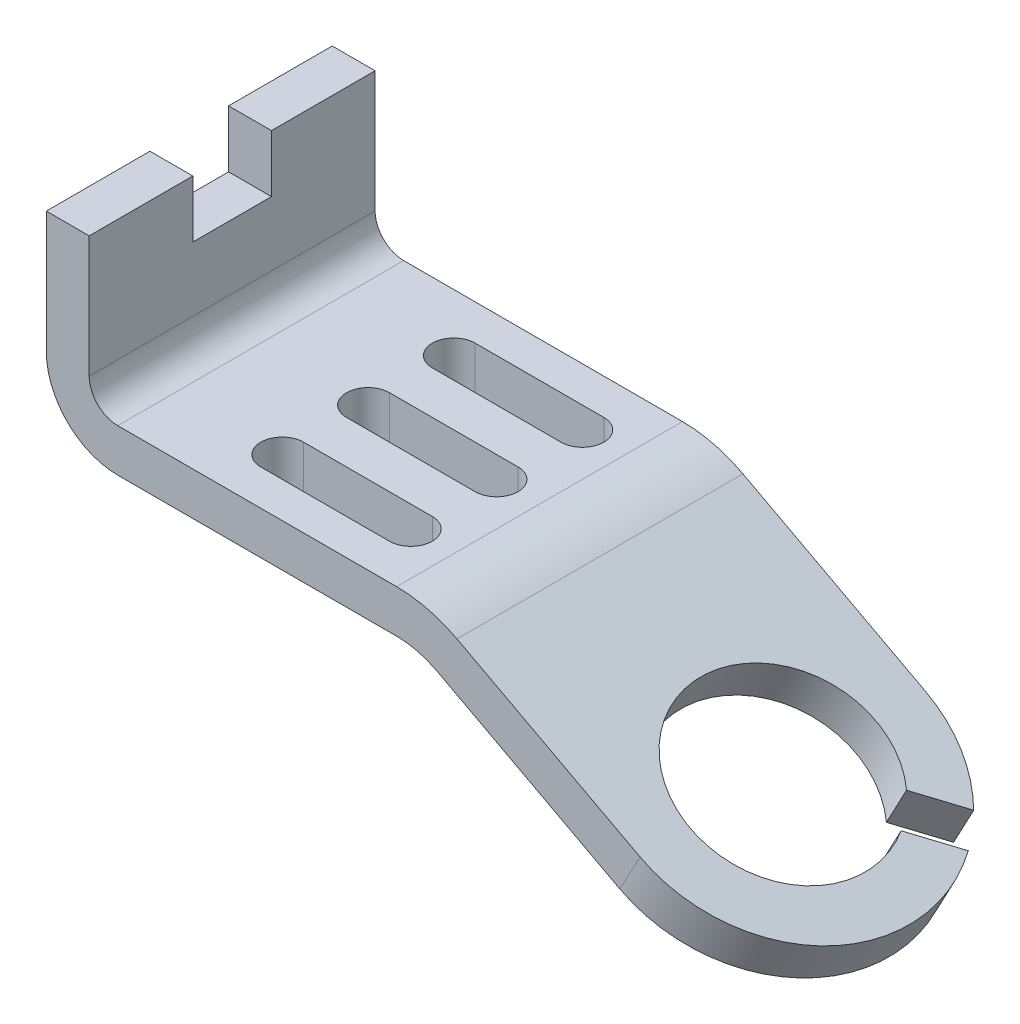
ISO-10303-21;
HEADER;
FILE_DESCRIPTION(('STEP AP214'),'2;1');
FILE_NAME('part.step','',(''),(''),'','','');
FILE_SCHEMA(('AUTOMOTIVE_DESIGN { 1 0 10303 214 1 1 1 1 }'));
ENDSEC;
DATA;
#1=APPLICATION_CONTEXT('core data for automotive mechanical design processes');
#2=APPLICATION_PROTOCOL_DEFINITION('international standard','automotive_design',2000,#1);
#3=PRODUCT_CONTEXT('',#1,'mechanical');
#4=PRODUCT('Part','Part','',(#3));
#5=PRODUCT_RELATED_PRODUCT_CATEGORY('part','',(#4));
#6=PRODUCT_DEFINITION_FORMATION('','',#4);
#7=PRODUCT_DEFINITION_CONTEXT('part definition',#1,'design');
#8=PRODUCT_DEFINITION('design','',#6,#7);
#9=PRODUCT_DEFINITION_SHAPE('','',#8);
#10=(LENGTH_UNIT() NAMED_UNIT(*) SI_UNIT(.MILLI.,.METRE.));
#11=(NAMED_UNIT(*) PLANE_ANGLE_UNIT() SI_UNIT($,.RADIAN.));
#12=(NAMED_UNIT(*) SI_UNIT($,.STERADIAN.) SOLID_ANGLE_UNIT());
#13=UNCERTAINTY_MEASURE_WITH_UNIT(LENGTH_MEASURE(1.E-05),#10,'distance_accuracy_value','');
#14=(GEOMETRIC_REPRESENTATION_CONTEXT(3) GLOBAL_UNCERTAINTY_ASSIGNED_CONTEXT((#13)) GLOBAL_UNIT_ASSIGNED_CONTEXT((#10,
#11,#12)) REPRESENTATION_CONTEXT('',''));
#15=CARTESIAN_POINT('',(0.,0.,0.));
#16=DIRECTION('',(0.,0.,1.));
#17=DIRECTION('',(1.,0.,0.));
#18=AXIS2_PLACEMENT_3D('',#15,#16,#17);
#19=CARTESIAN_POINT('',(0.,27.,40.));
#20=DIRECTION('',(0.,-1.,0.));
#21=DIRECTION('',(0.,0.,-1.));
#22=AXIS2_PLACEMENT_3D('',#19,#20,#21);
#23=PLANE('',#22);
#24=DIRECTION('',(0.,0.,-1.));
#25=VECTOR('',#24,1.);
#26=CARTESIAN_POINT('',(0.,27.,40.));
#27=LINE('',#26,#25);
#28=CARTESIAN_POINT('',(0.,27.,14.5));
#29=VERTEX_POINT('',#28);
#30=CARTESIAN_POINT('',(0.,27.,0.));
#31=VERTEX_POINT('',#30);
#32=EDGE_CURVE('E50',#29,#31,#27,.T.);
#33=ORIENTED_EDGE('',*,*,#32,.F.);
#34=DIRECTION('',(-1.,0.,0.));
#35=VECTOR('',#34,1.);
#36=CARTESIAN_POINT('',(-0.00100000000000013,27.,14.5));
#37=LINE('',#36,#35);
#38=CARTESIAN_POINT('',(6.,27.,14.5));
#39=VERTEX_POINT('',#38);
#40=EDGE_CURVE('E252',#39,#29,#37,.T.);
#41=ORIENTED_EDGE('',*,*,#40,.F.);
#42=DIRECTION('',(0.,0.,-1.));
#43=VECTOR('',#42,1.);
#44=CARTESIAN_POINT('',(6.,27.,40.));
#45=LINE('',#44,#43);
#46=CARTESIAN_POINT('',(6.,27.,0.));
#47=VERTEX_POINT('',#46);
#48=EDGE_CURVE('E264',#39,#47,#45,.T.);
#49=ORIENTED_EDGE('',*,*,#48,.T.);
#50=DIRECTION('',(-1.,0.,0.));
#51=VECTOR('',#50,1.);
#52=CARTESIAN_POINT('',(0.,27.,0.));
#53=LINE('',#52,#51);
#54=EDGE_CURVE('E312',#47,#31,#53,.T.);
#55=ORIENTED_EDGE('',*,*,#54,.T.);
#56=EDGE_LOOP('',(#33,#41,#49,#55));
#57=FACE_BOUND('',#56,.T.);
#58=ADVANCED_FACE('F39',(#57),#23,.F.);
#59=CARTESIAN_POINT('',(54.6417227193125,-1.40462888569289,40.));
#60=DIRECTION('',(0.469471562785892,0.882947592858927,0.));
#61=DIRECTION('',(-0.882947592858927,0.469471562785892,0.));
#62=AXIS2_PLACEMENT_3D('',#59,#60,#61);
#63=PLANE('',#62);
#64=CARTESIAN_POINT('',(80.2472029122214,-15.0193042064837,20.));
#65=DIRECTION('',(0.469471562785892,0.882947592858927,0.));
#66=DIRECTION('',(-0.882947592858927,0.469471562785892,0.));
#67=AXIS2_PLACEMENT_3D('',#64,#65,#66);
#68=CIRCLE('',#67,20.);
#69=CARTESIAN_POINT('',(94.7444514296889,-22.7276279763616,8.580213220838));
#70=VERTEX_POINT('',#69);
#71=CARTESIAN_POINT('',(80.2472029122214,-15.0193042064837,40.));
#72=VERTEX_POINT('',#71);
#73=EDGE_CURVE('E399',#70,#72,#68,.F.);
#74=ORIENTED_EDGE('',*,*,#73,.T.);
#75=DIRECTION('',(0.882947592858927,-0.469471562785892,0.));
#76=VECTOR('',#75,1.);
#77=CARTESIAN_POINT('',(54.6417227193125,-1.40462888569289,40.));
#78=LINE('',#77,#76);
#79=CARTESIAN_POINT('',(54.6417227193125,-1.40462888569288,40.));
#80=VERTEX_POINT('',#79);
#81=EDGE_CURVE('E358',#80,#72,#78,.T.);
#82=ORIENTED_EDGE('',*,*,#81,.F.);
#83=DIRECTION('',(0.,0.,-1.));
#84=VECTOR('',#83,1.);
#85=CARTESIAN_POINT('',(54.6417227193125,-1.40462888569288,40.));
#86=LINE('',#85,#84);
#87=CARTESIAN_POINT('',(54.6417227193125,-1.40462888569288,0.));
#88=VERTEX_POINT('',#87);
#89=EDGE_CURVE('E294',#80,#88,#86,.T.);
#90=ORIENTED_EDGE('',*,*,#89,.T.);
#91=DIRECTION('',(0.882947592858927,-0.469471562785892,0.));
#92=VECTOR('',#91,1.);
#93=CARTESIAN_POINT('',(54.6417227193125,-1.40462888569289,0.));
#94=LINE('',#93,#92);
#95=CARTESIAN_POINT('',(80.2472029122214,-15.0193042064837,0.));
#96=VERTEX_POINT('',#95);
#97=EDGE_CURVE('E332',#88,#96,#94,.T.);
#98=ORIENTED_EDGE('',*,*,#97,.T.);
#99=CARTESIAN_POINT('',(80.2472029122214,-15.0193042064837,20.));
#100=DIRECTION('',(0.469471562785892,0.882947592858927,0.));
#101=DIRECTION('',(-0.882947592858927,0.469471562785892,0.));
#102=AXIS2_PLACEMENT_3D('',#99,#100,#101);
#103=CIRCLE('',#102,20.);
#104=CARTESIAN_POINT('',(91.7904151387249,-21.1569390189858,4.86448909345104));
#105=VERTEX_POINT('',#104);
#106=EDGE_CURVE('E64',#96,#105,#103,.F.);
#107=ORIENTED_EDGE('',*,*,#106,.T.);
#108=DIRECTION('',(-0.656157934800832,0.34888536259312,0.669130606358859));
#109=VECTOR('',#108,1.);
#110=CARTESIAN_POINT('',(49.5631238493171,1.29571003310903,47.9266415521427));
#111=LINE('',#110,#109);
#112=CARTESIAN_POINT('',(87.1410217357462,-18.6848126951173,9.60580404513316));
#113=VERTEX_POINT('',#112);
#114=EDGE_CURVE('E835',#105,#113,#111,.T.);
#115=ORIENTED_EDGE('',*,*,#114,.T.);
#116=CARTESIAN_POINT('',(80.2472029122214,-15.0193042064837,20.));
#117=DIRECTION('',(0.469471562785892,0.882947592858927,0.));
#118=DIRECTION('',(-0.882947592858927,0.469471562785892,0.));
#119=AXIS2_PLACEMENT_3D('',#116,#117,#118);
#120=CIRCLE('',#119,13.);
#121=CARTESIAN_POINT('',(90.0950580267101,-20.2555016524931,13.3215281725201));
#122=VERTEX_POINT('',#121);
#123=EDGE_CURVE('E407',#122,#113,#120,.F.);
#124=ORIENTED_EDGE('',*,*,#123,.F.);
#125=DIRECTION('',(-0.65615793480083,0.34888536259312,0.669130606358861));
#126=VECTOR('',#125,1.);
#127=CARTESIAN_POINT('',(52.5171601402812,-0.274978924266915,51.6423656795297));
#128=LINE('',#127,#126);
#129=EDGE_CURVE('E402',#70,#122,#128,.T.);
#130=ORIENTED_EDGE('',*,*,#129,.F.);
#131=EDGE_LOOP('',(#74,#82,#90,#98,#107,#115,#124,#130));
#132=FACE_BOUND('',#131,.T.);
#133=ADVANCED_FACE('F395',(#132),#63,.F.);
#134=CARTESIAN_POINT('',(57.4585520960279,3.89305667146068,40.));
#135=DIRECTION('',(-0.469471562785892,-0.882947592858927,0.));
#136=DIRECTION('',(0.882947592858926,-0.469471562785892,0.));
#137=AXIS2_PLACEMENT_3D('',#134,#135,#136);
#138=PLANE('',#137);
#139=CARTESIAN_POINT('',(83.0640322889367,-9.72161864933019,20.));
#140=DIRECTION('',(0.469471562785892,0.882947592858926,0.));
#141=DIRECTION('',(-0.882947592858927,0.469471562785892,0.));
#142=AXIS2_PLACEMENT_3D('',#139,#140,#141);
#143=CIRCLE('',#142,20.);
#144=CARTESIAN_POINT('',(83.0640322889367,-9.72161864933019,40.));
#145=VERTEX_POINT('',#144);
#146=CARTESIAN_POINT('',(97.5612808064042,-17.4299424192081,8.58021322083801));
#147=VERTEX_POINT('',#146);
#148=EDGE_CURVE('E401',#145,#147,#143,.T.);
#149=ORIENTED_EDGE('',*,*,#148,.T.);
#150=DIRECTION('',(0.65615793480083,-0.34888536259312,-0.669130606358861));
#151=VECTOR('',#150,1.);
#152=CARTESIAN_POINT('',(55.3339895169966,5.02270663288664,51.6423656795296));
#153=LINE('',#152,#151);
#154=CARTESIAN_POINT('',(92.9118874034255,-14.9578160953396,13.3215281725201));
#155=VERTEX_POINT('',#154);
#156=EDGE_CURVE('E416',#155,#147,#153,.T.);
#157=ORIENTED_EDGE('',*,*,#156,.F.);
#158=CARTESIAN_POINT('',(83.0640322889367,-9.72161864933019,20.));
#159=DIRECTION('',(0.469471562785892,0.882947592858926,0.));
#160=DIRECTION('',(-0.882947592858927,0.469471562785892,0.));
#161=AXIS2_PLACEMENT_3D('',#158,#159,#160);
#162=CIRCLE('',#161,13.);
#163=CARTESIAN_POINT('',(89.9578511124615,-13.3871271379638,9.60580404513316));
#164=VERTEX_POINT('',#163);
#165=EDGE_CURVE('E415',#164,#155,#162,.T.);
#166=ORIENTED_EDGE('',*,*,#165,.F.);
#167=DIRECTION('',(0.656157934800832,-0.348885362593121,-0.669130606358859));
#168=VECTOR('',#167,1.);
#169=CARTESIAN_POINT('',(52.3799532260324,6.59339559026258,47.9266415521427));
#170=LINE('',#169,#168);
#171=CARTESIAN_POINT('',(94.6072445154403,-15.8592534618322,4.86448909345104));
#172=VERTEX_POINT('',#171);
#173=EDGE_CURVE('E412',#164,#172,#170,.T.);
#174=ORIENTED_EDGE('',*,*,#173,.T.);
#175=CARTESIAN_POINT('',(83.0640322889367,-9.72161864933019,0.));
#176=VERTEX_POINT('',#175);
#177=EDGE_CURVE('E408',#172,#176,#143,.T.);
#178=ORIENTED_EDGE('',*,*,#177,.T.);
#179=DIRECTION('',(-0.882947592858927,0.469471562785892,0.));
#180=VECTOR('',#179,1.);
#181=CARTESIAN_POINT('',(57.4585520960279,3.89305667146068,0.));
#182=LINE('',#181,#180);
#183=CARTESIAN_POINT('',(57.4585520960279,3.89305667146068,0.));
#184=VERTEX_POINT('',#183);
#185=EDGE_CURVE('E331',#176,#184,#182,.T.);
#186=ORIENTED_EDGE('',*,*,#185,.T.);
#187=DIRECTION('',(0.,0.,-1.));
#188=VECTOR('',#187,1.);
#189=CARTESIAN_POINT('',(57.4585520960279,3.89305667146068,40.));
#190=LINE('',#189,#188);
#191=CARTESIAN_POINT('',(57.4585520960279,3.89305667146068,40.));
#192=VERTEX_POINT('',#191);
#193=EDGE_CURVE('E292',#192,#184,#190,.T.);
#194=ORIENTED_EDGE('',*,*,#193,.F.);
#195=DIRECTION('',(-0.882947592858927,0.469471562785892,0.));
#196=VECTOR('',#195,1.);
#197=CARTESIAN_POINT('',(57.4585520960279,3.89305667146068,40.));
#198=LINE('',#197,#196);
#199=EDGE_CURVE('E362',#145,#192,#198,.T.);
#200=ORIENTED_EDGE('',*,*,#199,.F.);
#201=EDGE_LOOP('',(#149,#157,#166,#174,#178,#186,#194,#200));
#202=FACE_BOUND('',#201,.T.);
#203=ADVANCED_FACE('F553',(#202),#138,.F.);
#204=CARTESIAN_POINT('',(10.,10.,40.));
#205=DIRECTION('',(0.,0.,1.));
#206=DIRECTION('',(1.,0.,0.));
#207=AXIS2_PLACEMENT_3D('',#204,#205,#206);
#208=PLANE('',#207);
#209=ORIENTED_EDGE('',*,*,#81,.T.);
#210=DIRECTION('',(0.469471562785892,0.882947592858926,0.));
#211=VECTOR('',#210,1.);
#212=CARTESIAN_POINT('',(57.7654060668948,-57.3014145220289,40.));
#213=LINE('',#212,#211);
#214=EDGE_CURVE('E388',#72,#145,#213,.T.);
#215=ORIENTED_EDGE('',*,*,#214,.T.);
#216=ORIENTED_EDGE('',*,*,#199,.T.);
#217=CARTESIAN_POINT('',(49.0080639658818,-12.,40.));
#218=DIRECTION('',(0.,0.,1.));
#219=DIRECTION('',(-1.,0.,0.));
#220=AXIS2_PLACEMENT_3D('',#217,#218,#219);
#221=CIRCLE('',#220,18.);
#222=CARTESIAN_POINT('',(49.0080639658818,6.,40.));
#223=VERTEX_POINT('',#222);
#224=EDGE_CURVE('E365',#192,#223,#221,.T.);
#225=ORIENTED_EDGE('',*,*,#224,.T.);
#226=DIRECTION('',(-1.,0.,0.));
#227=VECTOR('',#226,1.);
#228=CARTESIAN_POINT('',(10.,6.,40.));
#229=LINE('',#228,#227);
#230=CARTESIAN_POINT('',(10.,6.,40.));
#231=VERTEX_POINT('',#230);
#232=EDGE_CURVE('E368',#223,#231,#229,.T.);
#233=ORIENTED_EDGE('',*,*,#232,.T.);
#234=CARTESIAN_POINT('',(10.,10.,40.));
#235=DIRECTION('',(0.,0.,-1.));
#236=DIRECTION('',(1.,0.,0.));
#237=AXIS2_PLACEMENT_3D('',#234,#235,#236);
#238=CIRCLE('',#237,4.);
#239=CARTESIAN_POINT('',(6.,10.0000000000001,40.));
#240=VERTEX_POINT('',#239);
#241=EDGE_CURVE('E276',#231,#240,#238,.T.);
#242=ORIENTED_EDGE('',*,*,#241,.T.);
#243=DIRECTION('',(0.,1.,0.));
#244=VECTOR('',#243,1.);
#245=CARTESIAN_POINT('',(6.,27.,40.));
#246=LINE('',#245,#244);
#247=CARTESIAN_POINT('',(6.,27.,40.));
#248=VERTEX_POINT('',#247);
#249=EDGE_CURVE('E274',#240,#248,#246,.T.);
#250=ORIENTED_EDGE('',*,*,#249,.T.);
#251=DIRECTION('',(-1.,0.,0.));
#252=VECTOR('',#251,1.);
#253=CARTESIAN_POINT('',(0.,27.,40.));
#254=LINE('',#253,#252);
#255=CARTESIAN_POINT('',(0.,27.,40.));
#256=VERTEX_POINT('',#255);
#257=EDGE_CURVE('E344',#248,#256,#254,.T.);
#258=ORIENTED_EDGE('',*,*,#257,.T.);
#259=DIRECTION('',(0.,-1.,0.));
#260=VECTOR('',#259,1.);
#261=CARTESIAN_POINT('',(0.,27.,40.));
#262=LINE('',#261,#260);
#263=CARTESIAN_POINT('',(0.,10.0000000000001,40.));
#264=VERTEX_POINT('',#263);
#265=EDGE_CURVE('E345',#256,#264,#262,.T.);
#266=ORIENTED_EDGE('',*,*,#265,.T.);
#267=CARTESIAN_POINT('',(10.,10.,40.));
#268=DIRECTION('',(0.,0.,1.));
#269=DIRECTION('',(1.,0.,0.));
#270=AXIS2_PLACEMENT_3D('',#267,#268,#269);
#271=CIRCLE('',#270,10.);
#272=CARTESIAN_POINT('',(10.0000000000001,0.,40.));
#273=VERTEX_POINT('',#272);
#274=EDGE_CURVE('E348',#264,#273,#271,.T.);
#275=ORIENTED_EDGE('',*,*,#274,.T.);
#276=DIRECTION('',(1.,0.,0.));
#277=VECTOR('',#276,1.);
#278=CARTESIAN_POINT('',(10.0000000000001,0.,40.));
#279=LINE('',#278,#277);
#280=CARTESIAN_POINT('',(49.0080639658818,0.,40.));
#281=VERTEX_POINT('',#280);
#282=EDGE_CURVE('E351',#273,#281,#279,.T.);
#283=ORIENTED_EDGE('',*,*,#282,.T.);
#284=CARTESIAN_POINT('',(49.0080639658818,-12.,40.));
#285=DIRECTION('',(0.,0.,-1.));
#286=DIRECTION('',(-1.,0.,0.));
#287=AXIS2_PLACEMENT_3D('',#284,#285,#286);
#288=CIRCLE('',#287,12.);
#289=EDGE_CURVE('E357',#281,#80,#288,.T.);
#290=ORIENTED_EDGE('',*,*,#289,.T.);
#291=EDGE_LOOP('',(#209,#215,#216,#225,#233,#242,#250,#258,#266,#275,#283,#290));
#292=FACE_BOUND('',#291,.T.);
#293=ADVANCED_FACE('F366',(#292),#208,.T.);
#294=CARTESIAN_POINT('',(10.,10.,0.));
#295=DIRECTION('',(0.,0.,1.));
#296=DIRECTION('',(1.,0.,0.));
#297=AXIS2_PLACEMENT_3D('',#294,#295,#296);
#298=PLANE('',#297);
#299=DIRECTION('',(0.469471562785892,0.882947592858926,0.));
#300=VECTOR('',#299,1.);
#301=CARTESIAN_POINT('',(57.7654060668948,-57.3014145220289,0.));
#302=LINE('',#301,#300);
#303=EDGE_CURVE('E429',#96,#176,#302,.T.);
#304=ORIENTED_EDGE('',*,*,#303,.F.);
#305=ORIENTED_EDGE('',*,*,#97,.F.);
#306=CARTESIAN_POINT('',(49.0080639658818,-12.,0.));
#307=DIRECTION('',(0.,0.,-1.));
#308=DIRECTION('',(-1.,0.,0.));
#309=AXIS2_PLACEMENT_3D('',#306,#307,#308);
#310=CIRCLE('',#309,12.);
#311=CARTESIAN_POINT('',(49.0080639658818,0.,0.));
#312=VERTEX_POINT('',#311);
#313=EDGE_CURVE('E328',#312,#88,#310,.T.);
#314=ORIENTED_EDGE('',*,*,#313,.F.);
#315=DIRECTION('',(1.,0.,0.));
#316=VECTOR('',#315,1.);
#317=CARTESIAN_POINT('',(10.0000000000001,0.,0.));
#318=LINE('',#317,#316);
#319=CARTESIAN_POINT('',(10.0000000000001,0.,0.));
#320=VERTEX_POINT('',#319);
#321=EDGE_CURVE('E330',#320,#312,#318,.T.);
#322=ORIENTED_EDGE('',*,*,#321,.F.);
#323=CARTESIAN_POINT('',(10.,10.,0.));
#324=DIRECTION('',(0.,0.,1.));
#325=DIRECTION('',(1.,0.,0.));
#326=AXIS2_PLACEMENT_3D('',#323,#324,#325);
#327=CIRCLE('',#326,10.);
#328=CARTESIAN_POINT('',(0.,10.0000000000001,0.));
#329=VERTEX_POINT('',#328);
#330=EDGE_CURVE('E320',#329,#320,#327,.T.);
#331=ORIENTED_EDGE('',*,*,#330,.F.);
#332=DIRECTION('',(0.,-1.,0.));
#333=VECTOR('',#332,1.);
#334=CARTESIAN_POINT('',(0.,27.,0.));
#335=LINE('',#334,#333);
#336=EDGE_CURVE('E315',#31,#329,#335,.T.);
#337=ORIENTED_EDGE('',*,*,#336,.F.);
#338=ORIENTED_EDGE('',*,*,#54,.F.);
#339=DIRECTION('',(0.,1.,0.));
#340=VECTOR('',#339,1.);
#341=CARTESIAN_POINT('',(6.,27.,0.));
#342=LINE('',#341,#340);
#343=CARTESIAN_POINT('',(6.,10.0000000000001,0.));
#344=VERTEX_POINT('',#343);
#345=EDGE_CURVE('E275',#344,#47,#342,.T.);
#346=ORIENTED_EDGE('',*,*,#345,.F.);
#347=CARTESIAN_POINT('',(10.,10.,0.));
#348=DIRECTION('',(0.,0.,-1.));
#349=DIRECTION('',(1.,0.,0.));
#350=AXIS2_PLACEMENT_3D('',#347,#348,#349);
#351=CIRCLE('',#350,4.);
#352=CARTESIAN_POINT('',(10.,6.,0.));
#353=VERTEX_POINT('',#352);
#354=EDGE_CURVE('E340',#353,#344,#351,.T.);
#355=ORIENTED_EDGE('',*,*,#354,.F.);
#356=DIRECTION('',(-1.,0.,0.));
#357=VECTOR('',#356,1.);
#358=CARTESIAN_POINT('',(10.,6.,0.));
#359=LINE('',#358,#357);
#360=CARTESIAN_POINT('',(49.0080639658818,6.,0.));
#361=VERTEX_POINT('',#360);
#362=EDGE_CURVE('E337',#361,#353,#359,.T.);
#363=ORIENTED_EDGE('',*,*,#362,.F.);
#364=CARTESIAN_POINT('',(49.0080639658818,-12.,0.));
#365=DIRECTION('',(0.,0.,1.));
#366=DIRECTION('',(-1.,0.,0.));
#367=AXIS2_PLACEMENT_3D('',#364,#365,#366);
#368=CIRCLE('',#367,18.);
#369=EDGE_CURVE('E338',#184,#361,#368,.T.);
#370=ORIENTED_EDGE('',*,*,#369,.F.);
#371=ORIENTED_EDGE('',*,*,#185,.F.);
#372=EDGE_LOOP('',(#304,#305,#314,#322,#331,#337,#338,#346,#355,#363,#370,#371));
#373=FACE_BOUND('',#372,.T.);
#374=ADVANCED_FACE('F314',(#373),#298,.F.);
#375=CARTESIAN_POINT('',(6.,27.,25.5));
#376=VERTEX_POINT('',#375);
#377=EDGE_CURVE('E273',#248,#376,#45,.T.);
#378=ORIENTED_EDGE('',*,*,#377,.T.);
#379=DIRECTION('',(1.,0.,0.));
#380=VECTOR('',#379,1.);
#381=CARTESIAN_POINT('',(-0.00100000000000013,27.,25.5));
#382=LINE('',#381,#380);
#383=CARTESIAN_POINT('',(0.,27.,25.5));
#384=VERTEX_POINT('',#383);
#385=EDGE_CURVE('E53',#384,#376,#382,.T.);
#386=ORIENTED_EDGE('',*,*,#385,.F.);
#387=EDGE_CURVE('E11',#256,#384,#27,.T.);
#388=ORIENTED_EDGE('',*,*,#387,.F.);
#389=ORIENTED_EDGE('',*,*,#257,.F.);
#390=EDGE_LOOP('',(#378,#386,#388,#389));
#391=FACE_BOUND('',#390,.T.);
#392=ADVANCED_FACE('F41',(#391),#23,.F.);
#393=CARTESIAN_POINT('',(0.,27.,40.));
#394=DIRECTION('',(1.,0.,0.));
#395=DIRECTION('',(0.,0.,-1.));
#396=AXIS2_PLACEMENT_3D('',#393,#394,#395);
#397=PLANE('',#396);
#398=DIRECTION('',(0.,0.,1.));
#399=VECTOR('',#398,1.);
#400=CARTESIAN_POINT('',(0.,19.,25.5));
#401=LINE('',#400,#399);
#402=CARTESIAN_POINT('',(0.,19.,14.5));
#403=VERTEX_POINT('',#402);
#404=CARTESIAN_POINT('',(0.,19.,25.5));
#405=VERTEX_POINT('',#404);
#406=EDGE_CURVE('E270',#403,#405,#401,.T.);
#407=ORIENTED_EDGE('',*,*,#406,.F.);
#408=DIRECTION('',(0.,-1.,0.));
#409=VECTOR('',#408,1.);
#410=CARTESIAN_POINT('',(0.,35.,14.5));
#411=LINE('',#410,#409);
#412=EDGE_CURVE('E257',#29,#403,#411,.T.);
#413=ORIENTED_EDGE('',*,*,#412,.F.);
#414=ORIENTED_EDGE('',*,*,#32,.T.);
#415=ORIENTED_EDGE('',*,*,#336,.T.);
#416=DIRECTION('',(0.,0.,-1.));
#417=VECTOR('',#416,1.);
#418=CARTESIAN_POINT('',(0.,10.0000000000001,40.));
#419=LINE('',#418,#417);
#420=EDGE_CURVE('E302',#264,#329,#419,.T.);
#421=ORIENTED_EDGE('',*,*,#420,.F.);
#422=ORIENTED_EDGE('',*,*,#265,.F.);
#423=ORIENTED_EDGE('',*,*,#387,.T.);
#424=DIRECTION('',(0.,1.,0.));
#425=VECTOR('',#424,1.);
#426=CARTESIAN_POINT('',(0.,35.,25.5));
#427=LINE('',#426,#425);
#428=EDGE_CURVE('E376',#405,#384,#427,.T.);
#429=ORIENTED_EDGE('',*,*,#428,.F.);
#430=EDGE_LOOP('',(#407,#413,#414,#415,#421,#422,#423,#429));
#431=FACE_BOUND('',#430,.T.);
#432=ADVANCED_FACE('F313',(#431),#397,.F.);
#433=CARTESIAN_POINT('',(10.,10.,40.));
#434=DIRECTION('',(0.,0.,-1.));
#435=DIRECTION('',(-1.,0.,0.));
#436=AXIS2_PLACEMENT_3D('',#433,#434,#435);
#437=CYLINDRICAL_SURFACE('',#436,10.);
#438=ORIENTED_EDGE('',*,*,#330,.T.);
#439=DIRECTION('',(0.,0.,-1.));
#440=VECTOR('',#439,1.);
#441=CARTESIAN_POINT('',(10.0000000000001,0.,40.));
#442=LINE('',#441,#440);
#443=EDGE_CURVE('E296',#273,#320,#442,.T.);
#444=ORIENTED_EDGE('',*,*,#443,.F.);
#445=ORIENTED_EDGE('',*,*,#274,.F.);
#446=ORIENTED_EDGE('',*,*,#420,.T.);
#447=EDGE_LOOP('',(#438,#444,#445,#446));
#448=FACE_BOUND('',#447,.T.);
#449=ADVANCED_FACE('F379',(#448),#437,.T.);
#450=CARTESIAN_POINT('',(10.0000000000001,0.,40.));
#451=DIRECTION('',(0.,1.,0.));
#452=DIRECTION('',(0.,0.,1.));
#453=AXIS2_PLACEMENT_3D('',#450,#451,#452);
#454=PLANE('',#453);
#455=DIRECTION('',(1.,0.,0.));
#456=VECTOR('',#455,1.);
#457=CARTESIAN_POINT('',(25.,0.,29.));
#458=LINE('',#457,#456);
#459=CARTESIAN_POINT('',(25.,0.,29.));
#460=VERTEX_POINT('',#459);
#461=CARTESIAN_POINT('',(43.,0.,29.));
#462=VERTEX_POINT('',#461);
#463=EDGE_CURVE('E467',#460,#462,#458,.T.);
#464=ORIENTED_EDGE('',*,*,#463,.F.);
#465=CARTESIAN_POINT('',(25.,0.,32.));
#466=DIRECTION('',(0.,1.,0.));
#467=DIRECTION('',(0.,0.,1.));
#468=AXIS2_PLACEMENT_3D('',#465,#466,#467);
#469=CIRCLE('',#468,3.);
#470=CARTESIAN_POINT('',(25.,0.,35.));
#471=VERTEX_POINT('',#470);
#472=EDGE_CURVE('E470',#471,#460,#469,.F.);
#473=ORIENTED_EDGE('',*,*,#472,.F.);
#474=DIRECTION('',(-1.,0.,0.));
#475=VECTOR('',#474,1.);
#476=CARTESIAN_POINT('',(25.,0.,35.));
#477=LINE('',#476,#475);
#478=CARTESIAN_POINT('',(43.,0.,35.));
#479=VERTEX_POINT('',#478);
#480=EDGE_CURVE('E436',#479,#471,#477,.T.);
#481=ORIENTED_EDGE('',*,*,#480,.F.);
#482=CARTESIAN_POINT('',(43.,0.,32.));
#483=DIRECTION('',(0.,1.,0.));
#484=DIRECTION('',(0.,0.,1.));
#485=AXIS2_PLACEMENT_3D('',#482,#483,#484);
#486=CIRCLE('',#485,3.);
#487=EDGE_CURVE('E421',#462,#479,#486,.F.);
#488=ORIENTED_EDGE('',*,*,#487,.F.);
#489=EDGE_LOOP('',(#464,#473,#481,#488));
#490=FACE_BOUND('',#489,.T.);
#491=DIRECTION('',(1.,0.,0.));
#492=VECTOR('',#491,1.);
#493=CARTESIAN_POINT('',(25.,0.,5.));
#494=LINE('',#493,#492);
#495=CARTESIAN_POINT('',(25.,0.,5.));
#496=VERTEX_POINT('',#495);
#497=CARTESIAN_POINT('',(43.,0.,5.));
#498=VERTEX_POINT('',#497);
#499=EDGE_CURVE('E434',#496,#498,#494,.T.);
#500=ORIENTED_EDGE('',*,*,#499,.F.);
#501=CARTESIAN_POINT('',(25.,0.,8.));
#502=DIRECTION('',(0.,1.,0.));
#503=DIRECTION('',(0.,0.,1.));
#504=AXIS2_PLACEMENT_3D('',#501,#502,#503);
#505=CIRCLE('',#504,3.);
#506=CARTESIAN_POINT('',(25.,0.,11.));
#507=VERTEX_POINT('',#506);
#508=EDGE_CURVE('E438',#507,#496,#505,.F.);
#509=ORIENTED_EDGE('',*,*,#508,.F.);
#510=DIRECTION('',(-1.,0.,0.));
#511=VECTOR('',#510,1.);
#512=CARTESIAN_POINT('',(25.,0.,11.));
#513=LINE('',#512,#511);
#514=CARTESIAN_POINT('',(43.,0.,11.));
#515=VERTEX_POINT('',#514);
#516=EDGE_CURVE('E457',#515,#507,#513,.T.);
#517=ORIENTED_EDGE('',*,*,#516,.F.);
#518=CARTESIAN_POINT('',(43.,0.,8.));
#519=DIRECTION('',(0.,1.,0.));
#520=DIRECTION('',(0.,0.,1.));
#521=AXIS2_PLACEMENT_3D('',#518,#519,#520);
#522=CIRCLE('',#521,3.);
#523=EDGE_CURVE('E433',#498,#515,#522,.F.);
#524=ORIENTED_EDGE('',*,*,#523,.F.);
#525=EDGE_LOOP('',(#500,#509,#517,#524));
#526=FACE_BOUND('',#525,.T.);
#527=DIRECTION('',(1.,0.,0.));
#528=VECTOR('',#527,1.);
#529=CARTESIAN_POINT('',(25.,0.,17.));
#530=LINE('',#529,#528);
#531=CARTESIAN_POINT('',(25.,0.,17.));
#532=VERTEX_POINT('',#531);
#533=CARTESIAN_POINT('',(43.,0.,17.));
#534=VERTEX_POINT('',#533);
#535=EDGE_CURVE('E497',#532,#534,#530,.T.);
#536=ORIENTED_EDGE('',*,*,#535,.F.);
#537=CARTESIAN_POINT('',(25.,0.,20.));
#538=DIRECTION('',(0.,1.,0.));
#539=DIRECTION('',(0.,0.,1.));
#540=AXIS2_PLACEMENT_3D('',#537,#538,#539);
#541=CIRCLE('',#540,3.);
#542=CARTESIAN_POINT('',(25.,0.,23.));
#543=VERTEX_POINT('',#542);
#544=EDGE_CURVE('E496',#543,#532,#541,.F.);
#545=ORIENTED_EDGE('',*,*,#544,.F.);
#546=DIRECTION('',(-1.,0.,0.));
#547=VECTOR('',#546,1.);
#548=CARTESIAN_POINT('',(25.,0.,23.));
#549=LINE('',#548,#547);
#550=CARTESIAN_POINT('',(43.,0.,23.));
#551=VERTEX_POINT('',#550);
#552=EDGE_CURVE('E317',#551,#543,#549,.T.);
#553=ORIENTED_EDGE('',*,*,#552,.F.);
#554=CARTESIAN_POINT('',(43.,0.,20.));
#555=DIRECTION('',(0.,1.,0.));
#556=DIRECTION('',(0.,0.,1.));
#557=AXIS2_PLACEMENT_3D('',#554,#555,#556);
#558=CIRCLE('',#557,3.);
#559=EDGE_CURVE('E461',#534,#551,#558,.F.);
#560=ORIENTED_EDGE('',*,*,#559,.F.);
#561=EDGE_LOOP('',(#536,#545,#553,#560));
#562=FACE_BOUND('',#561,.T.);
#563=ORIENTED_EDGE('',*,*,#321,.T.);
#564=DIRECTION('',(0.,0.,-1.));
#565=VECTOR('',#564,1.);
#566=CARTESIAN_POINT('',(49.0080639658818,0.,40.));
#567=LINE('',#566,#565);
#568=EDGE_CURVE('E299',#281,#312,#567,.T.);
#569=ORIENTED_EDGE('',*,*,#568,.F.);
#570=ORIENTED_EDGE('',*,*,#282,.F.);
#571=ORIENTED_EDGE('',*,*,#443,.T.);
#572=EDGE_LOOP('',(#563,#569,#570,#571));
#573=FACE_BOUND('',#572,.T.);
#574=ADVANCED_FACE('F385',(#490,#526,#562,#573),#454,.F.);
#575=CARTESIAN_POINT('',(49.0080639658818,-12.,40.));
#576=DIRECTION('',(0.,0.,-1.));
#577=DIRECTION('',(-1.,0.,0.));
#578=AXIS2_PLACEMENT_3D('',#575,#576,#577);
#579=CYLINDRICAL_SURFACE('',#578,12.);
#580=ORIENTED_EDGE('',*,*,#313,.T.);
#581=ORIENTED_EDGE('',*,*,#89,.F.);
#582=ORIENTED_EDGE('',*,*,#289,.F.);
#583=ORIENTED_EDGE('',*,*,#568,.T.);
#584=EDGE_LOOP('',(#580,#581,#582,#583));
#585=FACE_BOUND('',#584,.T.);
#586=ADVANCED_FACE('F390',(#585),#579,.F.);
#587=CARTESIAN_POINT('',(49.0080639658818,-12.,40.));
#588=DIRECTION('',(0.,0.,-1.));
#589=DIRECTION('',(-1.,0.,0.));
#590=AXIS2_PLACEMENT_3D('',#587,#588,#589);
#591=CYLINDRICAL_SURFACE('',#590,18.);
#592=ORIENTED_EDGE('',*,*,#369,.T.);
#593=DIRECTION('',(0.,0.,-1.));
#594=VECTOR('',#593,1.);
#595=CARTESIAN_POINT('',(49.0080639658818,6.,40.));
#596=LINE('',#595,#594);
#597=EDGE_CURVE('E289',#223,#361,#596,.T.);
#598=ORIENTED_EDGE('',*,*,#597,.F.);
#599=ORIENTED_EDGE('',*,*,#224,.F.);
#600=ORIENTED_EDGE('',*,*,#193,.T.);
#601=EDGE_LOOP('',(#592,#598,#599,#600));
#602=FACE_BOUND('',#601,.T.);
#603=ADVANCED_FACE('F575',(#602),#591,.T.);
#604=CARTESIAN_POINT('',(10.,6.,40.));
#605=DIRECTION('',(0.,-1.,0.));
#606=DIRECTION('',(1.,0.,0.));
#607=AXIS2_PLACEMENT_3D('',#604,#605,#606);
#608=PLANE('',#607);
#609=DIRECTION('',(1.,0.,0.));
#610=VECTOR('',#609,1.);
#611=CARTESIAN_POINT('',(25.,6.,35.));
#612=LINE('',#611,#610);
#613=CARTESIAN_POINT('',(25.,6.,35.));
#614=VERTEX_POINT('',#613);
#615=CARTESIAN_POINT('',(43.,6.,35.));
#616=VERTEX_POINT('',#615);
#617=EDGE_CURVE('E474',#614,#616,#612,.T.);
#618=ORIENTED_EDGE('',*,*,#617,.F.);
#619=CARTESIAN_POINT('',(25.,6.,32.));
#620=DIRECTION('',(0.,1.,0.));
#621=DIRECTION('',(-1.,0.,0.));
#622=AXIS2_PLACEMENT_3D('',#619,#620,#621);
#623=CIRCLE('',#622,3.);
#624=CARTESIAN_POINT('',(25.,6.,29.));
#625=VERTEX_POINT('',#624);
#626=EDGE_CURVE('E471',#625,#614,#623,.T.);
#627=ORIENTED_EDGE('',*,*,#626,.F.);
#628=DIRECTION('',(-1.,0.,0.));
#629=VECTOR('',#628,1.);
#630=CARTESIAN_POINT('',(25.,6.,29.));
#631=LINE('',#630,#629);
#632=CARTESIAN_POINT('',(43.,6.,29.));
#633=VERTEX_POINT('',#632);
#634=EDGE_CURVE('E481',#633,#625,#631,.T.);
#635=ORIENTED_EDGE('',*,*,#634,.F.);
#636=CARTESIAN_POINT('',(43.,6.,32.));
#637=DIRECTION('',(0.,1.,0.));
#638=DIRECTION('',(-1.,0.,0.));
#639=AXIS2_PLACEMENT_3D('',#636,#637,#638);
#640=CIRCLE('',#639,3.);
#641=EDGE_CURVE('E476',#616,#633,#640,.T.);
#642=ORIENTED_EDGE('',*,*,#641,.F.);
#643=EDGE_LOOP('',(#618,#627,#635,#642));
#644=FACE_BOUND('',#643,.T.);
#645=DIRECTION('',(1.,0.,0.));
#646=VECTOR('',#645,1.);
#647=CARTESIAN_POINT('',(25.,6.,11.));
#648=LINE('',#647,#646);
#649=CARTESIAN_POINT('',(25.,6.,11.));
#650=VERTEX_POINT('',#649);
#651=CARTESIAN_POINT('',(43.,6.,11.));
#652=VERTEX_POINT('',#651);
#653=EDGE_CURVE('E441',#650,#652,#648,.T.);
#654=ORIENTED_EDGE('',*,*,#653,.F.);
#655=CARTESIAN_POINT('',(25.,6.,8.));
#656=DIRECTION('',(0.,1.,0.));
#657=DIRECTION('',(-1.,0.,0.));
#658=AXIS2_PLACEMENT_3D('',#655,#656,#657);
#659=CIRCLE('',#658,3.);
#660=CARTESIAN_POINT('',(25.,6.,5.));
#661=VERTEX_POINT('',#660);
#662=EDGE_CURVE('E445',#661,#650,#659,.T.);
#663=ORIENTED_EDGE('',*,*,#662,.F.);
#664=DIRECTION('',(-1.,0.,0.));
#665=VECTOR('',#664,1.);
#666=CARTESIAN_POINT('',(25.,6.,5.));
#667=LINE('',#666,#665);
#668=CARTESIAN_POINT('',(43.,6.,5.));
#669=VERTEX_POINT('',#668);
#670=EDGE_CURVE('E446',#669,#661,#667,.T.);
#671=ORIENTED_EDGE('',*,*,#670,.F.);
#672=CARTESIAN_POINT('',(43.,6.,8.));
#673=DIRECTION('',(0.,1.,0.));
#674=DIRECTION('',(-1.,0.,0.));
#675=AXIS2_PLACEMENT_3D('',#672,#673,#674);
#676=CIRCLE('',#675,3.);
#677=EDGE_CURVE('E449',#652,#669,#676,.T.);
#678=ORIENTED_EDGE('',*,*,#677,.F.);
#679=EDGE_LOOP('',(#654,#663,#671,#678));
#680=FACE_BOUND('',#679,.T.);
#681=DIRECTION('',(1.,0.,0.));
#682=VECTOR('',#681,1.);
#683=CARTESIAN_POINT('',(25.,6.,23.));
#684=LINE('',#683,#682);
#685=CARTESIAN_POINT('',(25.,6.,23.));
#686=VERTEX_POINT('',#685);
#687=CARTESIAN_POINT('',(43.,6.,23.));
#688=VERTEX_POINT('',#687);
#689=EDGE_CURVE('E505',#686,#688,#684,.T.);
#690=ORIENTED_EDGE('',*,*,#689,.F.);
#691=CARTESIAN_POINT('',(25.,6.,20.));
#692=DIRECTION('',(0.,1.,0.));
#693=DIRECTION('',(-1.,0.,0.));
#694=AXIS2_PLACEMENT_3D('',#691,#692,#693);
#695=CIRCLE('',#694,3.);
#696=CARTESIAN_POINT('',(25.,6.,17.));
#697=VERTEX_POINT('',#696);
#698=EDGE_CURVE('E504',#697,#686,#695,.T.);
#699=ORIENTED_EDGE('',*,*,#698,.F.);
#700=DIRECTION('',(-1.,0.,0.));
#701=VECTOR('',#700,1.);
#702=CARTESIAN_POINT('',(25.,6.,17.));
#703=LINE('',#702,#701);
#704=CARTESIAN_POINT('',(43.,6.,17.));
#705=VERTEX_POINT('',#704);
#706=EDGE_CURVE('E510',#705,#697,#703,.T.);
#707=ORIENTED_EDGE('',*,*,#706,.F.);
#708=CARTESIAN_POINT('',(43.,6.,20.));
#709=DIRECTION('',(0.,1.,0.));
#710=DIRECTION('',(-1.,0.,0.));
#711=AXIS2_PLACEMENT_3D('',#708,#709,#710);
#712=CIRCLE('',#711,3.);
#713=EDGE_CURVE('E507',#688,#705,#712,.T.);
#714=ORIENTED_EDGE('',*,*,#713,.F.);
#715=EDGE_LOOP('',(#690,#699,#707,#714));
#716=FACE_BOUND('',#715,.T.);
#717=ORIENTED_EDGE('',*,*,#362,.T.);
#718=DIRECTION('',(0.,0.,-1.));
#719=VECTOR('',#718,1.);
#720=CARTESIAN_POINT('',(10.,6.,40.));
#721=LINE('',#720,#719);
#722=EDGE_CURVE('E281',#231,#353,#721,.T.);
#723=ORIENTED_EDGE('',*,*,#722,.F.);
#724=ORIENTED_EDGE('',*,*,#232,.F.);
#725=ORIENTED_EDGE('',*,*,#597,.T.);
#726=EDGE_LOOP('',(#717,#723,#724,#725));
#727=FACE_BOUND('',#726,.T.);
#728=ADVANCED_FACE('F530',(#644,#680,#716,#727),#608,.F.);
#729=CARTESIAN_POINT('',(10.,10.,40.));
#730=DIRECTION('',(0.,0.,-1.));
#731=DIRECTION('',(-1.,0.,0.));
#732=AXIS2_PLACEMENT_3D('',#729,#730,#731);
#733=CYLINDRICAL_SURFACE('',#732,4.);
#734=ORIENTED_EDGE('',*,*,#354,.T.);
#735=DIRECTION('',(0.,0.,-1.));
#736=VECTOR('',#735,1.);
#737=CARTESIAN_POINT('',(6.,10.0000000000001,40.));
#738=LINE('',#737,#736);
#739=EDGE_CURVE('E279',#240,#344,#738,.T.);
#740=ORIENTED_EDGE('',*,*,#739,.F.);
#741=ORIENTED_EDGE('',*,*,#241,.F.);
#742=ORIENTED_EDGE('',*,*,#722,.T.);
#743=EDGE_LOOP('',(#734,#740,#741,#742));
#744=FACE_BOUND('',#743,.T.);
#745=ADVANCED_FACE('F373',(#744),#733,.F.);
#746=CARTESIAN_POINT('',(6.,27.,40.));
#747=DIRECTION('',(-1.,0.,0.));
#748=DIRECTION('',(0.,0.,1.));
#749=AXIS2_PLACEMENT_3D('',#746,#747,#748);
#750=PLANE('',#749);
#751=ORIENTED_EDGE('',*,*,#48,.F.);
#752=DIRECTION('',(0.,1.,0.));
#753=VECTOR('',#752,1.);
#754=CARTESIAN_POINT('',(6.,35.,14.5));
#755=LINE('',#754,#753);
#756=CARTESIAN_POINT('',(6.,19.,14.5));
#757=VERTEX_POINT('',#756);
#758=EDGE_CURVE('E249',#757,#39,#755,.T.);
#759=ORIENTED_EDGE('',*,*,#758,.F.);
#760=DIRECTION('',(0.,0.,-1.));
#761=VECTOR('',#760,1.);
#762=CARTESIAN_POINT('',(6.,19.,25.5));
#763=LINE('',#762,#761);
#764=CARTESIAN_POINT('',(6.,19.,25.5));
#765=VERTEX_POINT('',#764);
#766=EDGE_CURVE('E829',#765,#757,#763,.T.);
#767=ORIENTED_EDGE('',*,*,#766,.F.);
#768=DIRECTION('',(0.,-1.,0.));
#769=VECTOR('',#768,1.);
#770=CARTESIAN_POINT('',(6.,35.,25.5));
#771=LINE('',#770,#769);
#772=EDGE_CURVE('E259',#376,#765,#771,.T.);
#773=ORIENTED_EDGE('',*,*,#772,.F.);
#774=ORIENTED_EDGE('',*,*,#377,.F.);
#775=ORIENTED_EDGE('',*,*,#249,.F.);
#776=ORIENTED_EDGE('',*,*,#739,.T.);
#777=ORIENTED_EDGE('',*,*,#345,.T.);
#778=EDGE_LOOP('',(#751,#759,#767,#773,#774,#775,#776,#777));
#779=FACE_BOUND('',#778,.T.);
#780=ADVANCED_FACE('F267',(#779),#750,.F.);
#781=CARTESIAN_POINT('',(25.,-26.586471583074,20.));
#782=DIRECTION('',(0.,1.,0.));
#783=DIRECTION('',(-1.,0.,0.));
#784=AXIS2_PLACEMENT_3D('',#781,#782,#783);
#785=CYLINDRICAL_SURFACE('',#784,3.);
#786=ORIENTED_EDGE('',*,*,#544,.T.);
#787=DIRECTION('',(0.,1.,0.));
#788=VECTOR('',#787,1.);
#789=CARTESIAN_POINT('',(25.,-26.586471583074,17.));
#790=LINE('',#789,#788);
#791=EDGE_CURVE('E325',#532,#697,#790,.T.);
#792=ORIENTED_EDGE('',*,*,#791,.T.);
#793=ORIENTED_EDGE('',*,*,#698,.T.);
#794=DIRECTION('',(0.,1.,0.));
#795=VECTOR('',#794,1.);
#796=CARTESIAN_POINT('',(25.,-26.586471583074,23.));
#797=LINE('',#796,#795);
#798=EDGE_CURVE('E511',#543,#686,#797,.T.);
#799=ORIENTED_EDGE('',*,*,#798,.F.);
#800=EDGE_LOOP('',(#786,#792,#793,#799));
#801=FACE_BOUND('',#800,.T.);
#802=ADVANCED_FACE('F540',(#801),#785,.F.);
#803=CARTESIAN_POINT('',(25.,-26.586471583074,17.));
#804=DIRECTION('',(0.,0.,-1.));
#805=DIRECTION('',(-1.,0.,0.));
#806=AXIS2_PLACEMENT_3D('',#803,#804,#805);
#807=PLANE('',#806);
#808=ORIENTED_EDGE('',*,*,#535,.T.);
#809=DIRECTION('',(0.,1.,0.));
#810=VECTOR('',#809,1.);
#811=CARTESIAN_POINT('',(43.,-26.586471583074,17.));
#812=LINE('',#811,#810);
#813=EDGE_CURVE('E513',#534,#705,#812,.T.);
#814=ORIENTED_EDGE('',*,*,#813,.T.);
#815=ORIENTED_EDGE('',*,*,#706,.T.);
#816=ORIENTED_EDGE('',*,*,#791,.F.);
#817=EDGE_LOOP('',(#808,#814,#815,#816));
#818=FACE_BOUND('',#817,.T.);
#819=ADVANCED_FACE('F537',(#818),#807,.F.);
#820=CARTESIAN_POINT('',(43.,-26.586471583074,20.));
#821=DIRECTION('',(0.,1.,0.));
#822=DIRECTION('',(-1.,0.,0.));
#823=AXIS2_PLACEMENT_3D('',#820,#821,#822);
#824=CYLINDRICAL_SURFACE('',#823,3.);
#825=ORIENTED_EDGE('',*,*,#559,.T.);
#826=DIRECTION('',(0.,1.,0.));
#827=VECTOR('',#826,1.);
#828=CARTESIAN_POINT('',(43.,-26.586471583074,23.));
#829=LINE('',#828,#827);
#830=EDGE_CURVE('E519',#551,#688,#829,.T.);
#831=ORIENTED_EDGE('',*,*,#830,.T.);
#832=ORIENTED_EDGE('',*,*,#713,.T.);
#833=ORIENTED_EDGE('',*,*,#813,.F.);
#834=EDGE_LOOP('',(#825,#831,#832,#833));
#835=FACE_BOUND('',#834,.T.);
#836=ADVANCED_FACE('F531',(#835),#824,.F.);
#837=CARTESIAN_POINT('',(25.,-26.586471583074,23.));
#838=DIRECTION('',(0.,0.,1.));
#839=DIRECTION('',(1.,0.,0.));
#840=AXIS2_PLACEMENT_3D('',#837,#838,#839);
#841=PLANE('',#840);
#842=ORIENTED_EDGE('',*,*,#552,.T.);
#843=ORIENTED_EDGE('',*,*,#798,.T.);
#844=ORIENTED_EDGE('',*,*,#689,.T.);
#845=ORIENTED_EDGE('',*,*,#830,.F.);
#846=EDGE_LOOP('',(#842,#843,#844,#845));
#847=FACE_BOUND('',#846,.T.);
#848=ADVANCED_FACE('F521',(#847),#841,.F.);
#849=CARTESIAN_POINT('',(25.,-26.586471583074,8.));
#850=DIRECTION('',(0.,1.,0.));
#851=DIRECTION('',(-1.,0.,0.));
#852=AXIS2_PLACEMENT_3D('',#849,#850,#851);
#853=CYLINDRICAL_SURFACE('',#852,3.);
#854=ORIENTED_EDGE('',*,*,#508,.T.);
#855=DIRECTION('',(0.,1.,0.));
#856=VECTOR('',#855,1.);
#857=CARTESIAN_POINT('',(25.,-26.586471583074,5.));
#858=LINE('',#857,#856);
#859=EDGE_CURVE('E453',#496,#661,#858,.T.);
#860=ORIENTED_EDGE('',*,*,#859,.T.);
#861=ORIENTED_EDGE('',*,*,#662,.T.);
#862=DIRECTION('',(0.,1.,0.));
#863=VECTOR('',#862,1.);
#864=CARTESIAN_POINT('',(25.,-26.586471583074,11.));
#865=LINE('',#864,#863);
#866=EDGE_CURVE('E454',#507,#650,#865,.T.);
#867=ORIENTED_EDGE('',*,*,#866,.F.);
#868=EDGE_LOOP('',(#854,#860,#861,#867));
#869=FACE_BOUND('',#868,.T.);
#870=ADVANCED_FACE('F642',(#869),#853,.F.);
#871=CARTESIAN_POINT('',(25.,-26.586471583074,5.));
#872=DIRECTION('',(0.,0.,-1.));
#873=DIRECTION('',(-1.,0.,0.));
#874=AXIS2_PLACEMENT_3D('',#871,#872,#873);
#875=PLANE('',#874);
#876=ORIENTED_EDGE('',*,*,#499,.T.);
#877=DIRECTION('',(0.,1.,0.));
#878=VECTOR('',#877,1.);
#879=CARTESIAN_POINT('',(43.,-26.586471583074,5.));
#880=LINE('',#879,#878);
#881=EDGE_CURVE('E460',#498,#669,#880,.T.);
#882=ORIENTED_EDGE('',*,*,#881,.T.);
#883=ORIENTED_EDGE('',*,*,#670,.T.);
#884=ORIENTED_EDGE('',*,*,#859,.F.);
#885=EDGE_LOOP('',(#876,#882,#883,#884));
#886=FACE_BOUND('',#885,.T.);
#887=ADVANCED_FACE('F652',(#886),#875,.F.);
#888=CARTESIAN_POINT('',(43.,-26.586471583074,8.));
#889=DIRECTION('',(0.,1.,0.));
#890=DIRECTION('',(-1.,0.,0.));
#891=AXIS2_PLACEMENT_3D('',#888,#889,#890);
#892=CYLINDRICAL_SURFACE('',#891,3.);
#893=ORIENTED_EDGE('',*,*,#523,.T.);
#894=DIRECTION('',(0.,1.,0.));
#895=VECTOR('',#894,1.);
#896=CARTESIAN_POINT('',(43.,-26.586471583074,11.));
#897=LINE('',#896,#895);
#898=EDGE_CURVE('E459',#515,#652,#897,.T.);
#899=ORIENTED_EDGE('',*,*,#898,.T.);
#900=ORIENTED_EDGE('',*,*,#677,.T.);
#901=ORIENTED_EDGE('',*,*,#881,.F.);
#902=EDGE_LOOP('',(#893,#899,#900,#901));
#903=FACE_BOUND('',#902,.T.);
#904=ADVANCED_FACE('F661',(#903),#892,.F.);
#905=CARTESIAN_POINT('',(25.,-26.586471583074,11.));
#906=DIRECTION('',(0.,0.,1.));
#907=DIRECTION('',(1.,0.,0.));
#908=AXIS2_PLACEMENT_3D('',#905,#906,#907);
#909=PLANE('',#908);
#910=ORIENTED_EDGE('',*,*,#516,.T.);
#911=ORIENTED_EDGE('',*,*,#866,.T.);
#912=ORIENTED_EDGE('',*,*,#653,.T.);
#913=ORIENTED_EDGE('',*,*,#898,.F.);
#914=EDGE_LOOP('',(#910,#911,#912,#913));
#915=FACE_BOUND('',#914,.T.);
#916=ADVANCED_FACE('F673',(#915),#909,.F.);
#917=CARTESIAN_POINT('',(25.,-26.586471583074,32.));
#918=DIRECTION('',(0.,1.,0.));
#919=DIRECTION('',(-1.,0.,0.));
#920=AXIS2_PLACEMENT_3D('',#917,#918,#919);
#921=CYLINDRICAL_SURFACE('',#920,3.);
#922=ORIENTED_EDGE('',*,*,#472,.T.);
#923=DIRECTION('',(0.,1.,0.));
#924=VECTOR('',#923,1.);
#925=CARTESIAN_POINT('',(25.,-26.586471583074,29.));
#926=LINE('',#925,#924);
#927=EDGE_CURVE('E484',#460,#625,#926,.T.);
#928=ORIENTED_EDGE('',*,*,#927,.T.);
#929=ORIENTED_EDGE('',*,*,#626,.T.);
#930=DIRECTION('',(0.,1.,0.));
#931=VECTOR('',#930,1.);
#932=CARTESIAN_POINT('',(25.,-26.586471583074,35.));
#933=LINE('',#932,#931);
#934=EDGE_CURVE('E482',#471,#614,#933,.T.);
#935=ORIENTED_EDGE('',*,*,#934,.F.);
#936=EDGE_LOOP('',(#922,#928,#929,#935));
#937=FACE_BOUND('',#936,.T.);
#938=ADVANCED_FACE('F685',(#937),#921,.F.);
#939=CARTESIAN_POINT('',(25.,-26.586471583074,29.));
#940=DIRECTION('',(0.,0.,-1.));
#941=DIRECTION('',(-1.,0.,0.));
#942=AXIS2_PLACEMENT_3D('',#939,#940,#941);
#943=PLANE('',#942);
#944=ORIENTED_EDGE('',*,*,#463,.T.);
#945=DIRECTION('',(0.,1.,0.));
#946=VECTOR('',#945,1.);
#947=CARTESIAN_POINT('',(43.,-26.586471583074,29.));
#948=LINE('',#947,#946);
#949=EDGE_CURVE('E490',#462,#633,#948,.T.);
#950=ORIENTED_EDGE('',*,*,#949,.T.);
#951=ORIENTED_EDGE('',*,*,#634,.T.);
#952=ORIENTED_EDGE('',*,*,#927,.F.);
#953=EDGE_LOOP('',(#944,#950,#951,#952));
#954=FACE_BOUND('',#953,.T.);
#955=ADVANCED_FACE('F695',(#954),#943,.F.);
#956=CARTESIAN_POINT('',(43.,-26.586471583074,32.));
#957=DIRECTION('',(0.,1.,0.));
#958=DIRECTION('',(-1.,0.,0.));
#959=AXIS2_PLACEMENT_3D('',#956,#957,#958);
#960=CYLINDRICAL_SURFACE('',#959,3.);
#961=ORIENTED_EDGE('',*,*,#487,.T.);
#962=DIRECTION('',(0.,1.,0.));
#963=VECTOR('',#962,1.);
#964=CARTESIAN_POINT('',(43.,-26.586471583074,35.));
#965=LINE('',#964,#963);
#966=EDGE_CURVE('E487',#479,#616,#965,.T.);
#967=ORIENTED_EDGE('',*,*,#966,.T.);
#968=ORIENTED_EDGE('',*,*,#641,.T.);
#969=ORIENTED_EDGE('',*,*,#949,.F.);
#970=EDGE_LOOP('',(#961,#967,#968,#969));
#971=FACE_BOUND('',#970,.T.);
#972=ADVANCED_FACE('F703',(#971),#960,.F.);
#973=CARTESIAN_POINT('',(25.,-26.586471583074,35.));
#974=DIRECTION('',(0.,0.,1.));
#975=DIRECTION('',(1.,0.,0.));
#976=AXIS2_PLACEMENT_3D('',#973,#974,#975);
#977=PLANE('',#976);
#978=ORIENTED_EDGE('',*,*,#480,.T.);
#979=ORIENTED_EDGE('',*,*,#934,.T.);
#980=ORIENTED_EDGE('',*,*,#617,.T.);
#981=ORIENTED_EDGE('',*,*,#966,.F.);
#982=EDGE_LOOP('',(#978,#979,#980,#981));
#983=FACE_BOUND('',#982,.T.);
#984=ADVANCED_FACE('F712',(#983),#977,.F.);
#985=CARTESIAN_POINT('',(57.7654060668948,-57.3014145220289,20.));
#986=DIRECTION('',(0.469471562785892,0.882947592858926,0.));
#987=DIRECTION('',(-0.882947592858927,0.469471562785892,0.));
#988=AXIS2_PLACEMENT_3D('',#985,#986,#987);
#989=CYLINDRICAL_SURFACE('',#988,20.);
#990=DIRECTION('',(0.469471562785892,0.882947592858926,0.));
#991=VECTOR('',#990,1.);
#992=CARTESIAN_POINT('',(72.2626545843623,-65.0097382919068,8.58021322083801));
#993=LINE('',#992,#991);
#994=EDGE_CURVE('E423',#70,#147,#993,.T.);
#995=ORIENTED_EDGE('',*,*,#994,.T.);
#996=ORIENTED_EDGE('',*,*,#148,.F.);
#997=ORIENTED_EDGE('',*,*,#214,.F.);
#998=ORIENTED_EDGE('',*,*,#73,.F.);
#999=EDGE_LOOP('',(#995,#996,#997,#998));
#1000=FACE_BOUND('',#999,.T.);
#1001=ADVANCED_FACE('F722',(#1000),#989,.T.);
#1002=CARTESIAN_POINT('',(30.0353632949547,-42.5570892398121,51.6423656795296));
#1003=DIRECTION('',(0.59080725819279,-0.314137791475166,0.743144825477391));
#1004=DIRECTION('',(0.782770714089815,0.,-0.622310219394894));
#1005=AXIS2_PLACEMENT_3D('',#1002,#1003,#1004);
#1006=PLANE('',#1005);
#1007=ORIENTED_EDGE('',*,*,#129,.T.);
#1008=DIRECTION('',(0.469471562785892,0.882947592858926,0.));
#1009=VECTOR('',#1008,1.);
#1010=CARTESIAN_POINT('',(67.6132611813836,-62.5376119680384,13.3215281725201));
#1011=LINE('',#1010,#1009);
#1012=EDGE_CURVE('E424',#122,#155,#1011,.T.);
#1013=ORIENTED_EDGE('',*,*,#1012,.T.);
#1014=ORIENTED_EDGE('',*,*,#156,.T.);
#1015=ORIENTED_EDGE('',*,*,#994,.F.);
#1016=EDGE_LOOP('',(#1007,#1013,#1014,#1015));
#1017=FACE_BOUND('',#1016,.T.);
#1018=ADVANCED_FACE('F753',(#1017),#1006,.F.);
#1019=CARTESIAN_POINT('',(57.7654060668948,-57.3014145220289,20.));
#1020=DIRECTION('',(0.469471562785892,0.882947592858926,0.));
#1021=DIRECTION('',(-0.882947592858927,0.469471562785892,0.));
#1022=AXIS2_PLACEMENT_3D('',#1019,#1020,#1021);
#1023=CYLINDRICAL_SURFACE('',#1022,13.);
#1024=ORIENTED_EDGE('',*,*,#123,.T.);
#1025=DIRECTION('',(0.469471562785892,0.882947592858926,0.));
#1026=VECTOR('',#1025,1.);
#1027=CARTESIAN_POINT('',(64.6592248904196,-60.9669230106625,9.60580404513316));
#1028=LINE('',#1027,#1026);
#1029=EDGE_CURVE('E426',#113,#164,#1028,.T.);
#1030=ORIENTED_EDGE('',*,*,#1029,.T.);
#1031=ORIENTED_EDGE('',*,*,#165,.T.);
#1032=ORIENTED_EDGE('',*,*,#1012,.F.);
#1033=EDGE_LOOP('',(#1024,#1030,#1031,#1032));
#1034=FACE_BOUND('',#1033,.T.);
#1035=ADVANCED_FACE('F761',(#1034),#1023,.F.);
#1036=CARTESIAN_POINT('',(27.0813270039905,-40.9864002824362,47.9266415521427));
#1037=DIRECTION('',(0.590807258192789,-0.314137791475165,0.743144825477393));
#1038=DIRECTION('',(0.782770714089816,0.,-0.622310219394892));
#1039=AXIS2_PLACEMENT_3D('',#1036,#1037,#1038);
#1040=PLANE('',#1039);
#1041=DIRECTION('',(0.469471562785892,0.882947592858926,0.));
#1042=VECTOR('',#1041,1.);
#1043=CARTESIAN_POINT('',(69.3086182933984,-63.439049334531,4.86448909345104));
#1044=LINE('',#1043,#1042);
#1045=EDGE_CURVE('E428',#105,#172,#1044,.T.);
#1046=ORIENTED_EDGE('',*,*,#1045,.T.);
#1047=ORIENTED_EDGE('',*,*,#173,.F.);
#1048=ORIENTED_EDGE('',*,*,#1029,.F.);
#1049=ORIENTED_EDGE('',*,*,#114,.F.);
#1050=EDGE_LOOP('',(#1046,#1047,#1048,#1049));
#1051=FACE_BOUND('',#1050,.T.);
#1052=ADVANCED_FACE('F772',(#1051),#1040,.T.);
#1053=ORIENTED_EDGE('',*,*,#303,.T.);
#1054=ORIENTED_EDGE('',*,*,#177,.F.);
#1055=ORIENTED_EDGE('',*,*,#1045,.F.);
#1056=ORIENTED_EDGE('',*,*,#106,.F.);
#1057=EDGE_LOOP('',(#1053,#1054,#1055,#1056));
#1058=FACE_BOUND('',#1057,.T.);
#1059=ADVANCED_FACE('F751',(#1058),#989,.T.);
#1060=CARTESIAN_POINT('',(-0.00100000000000013,35.,14.5));
#1061=DIRECTION('',(0.,0.,-1.));
#1062=DIRECTION('',(0.,1.,0.));
#1063=AXIS2_PLACEMENT_3D('',#1060,#1061,#1062);
#1064=PLANE('',#1063);
#1065=ORIENTED_EDGE('',*,*,#40,.T.);
#1066=ORIENTED_EDGE('',*,*,#412,.T.);
#1067=DIRECTION('',(1.,0.,0.));
#1068=VECTOR('',#1067,1.);
#1069=CARTESIAN_POINT('',(-0.00100000000000013,19.,14.5));
#1070=LINE('',#1069,#1068);
#1071=EDGE_CURVE('E255',#403,#757,#1070,.T.);
#1072=ORIENTED_EDGE('',*,*,#1071,.T.);
#1073=ORIENTED_EDGE('',*,*,#758,.T.);
#1074=EDGE_LOOP('',(#1065,#1066,#1072,#1073));
#1075=FACE_BOUND('',#1074,.T.);
#1076=ADVANCED_FACE('F250',(#1075),#1064,.F.);
#1077=CARTESIAN_POINT('',(-0.00100000000000013,19.,25.5));
#1078=DIRECTION('',(0.,-1.,0.));
#1079=DIRECTION('',(0.,0.,-1.));
#1080=AXIS2_PLACEMENT_3D('',#1077,#1078,#1079);
#1081=PLANE('',#1080);
#1082=ORIENTED_EDGE('',*,*,#406,.T.);
#1083=DIRECTION('',(1.,0.,0.));
#1084=VECTOR('',#1083,1.);
#1085=CARTESIAN_POINT('',(-0.00100000000000013,19.,25.5));
#1086=LINE('',#1085,#1084);
#1087=EDGE_CURVE('E825',#405,#765,#1086,.T.);
#1088=ORIENTED_EDGE('',*,*,#1087,.T.);
#1089=ORIENTED_EDGE('',*,*,#766,.T.);
#1090=ORIENTED_EDGE('',*,*,#1071,.F.);
#1091=EDGE_LOOP('',(#1082,#1088,#1089,#1090));
#1092=FACE_BOUND('',#1091,.T.);
#1093=ADVANCED_FACE('F800',(#1092),#1081,.F.);
#1094=CARTESIAN_POINT('',(-0.00100000000000013,35.,25.5));
#1095=DIRECTION('',(0.,0.,1.));
#1096=DIRECTION('',(1.,0.,0.));
#1097=AXIS2_PLACEMENT_3D('',#1094,#1095,#1096);
#1098=PLANE('',#1097);
#1099=ORIENTED_EDGE('',*,*,#385,.T.);
#1100=ORIENTED_EDGE('',*,*,#772,.T.);
#1101=ORIENTED_EDGE('',*,*,#1087,.F.);
#1102=ORIENTED_EDGE('',*,*,#428,.T.);
#1103=EDGE_LOOP('',(#1099,#1100,#1101,#1102));
#1104=FACE_BOUND('',#1103,.T.);
#1105=ADVANCED_FACE('F809',(#1104),#1098,.F.);
#1106=CLOSED_SHELL('',(#58,#133,#203,#293,#374,#392,#432,#449,#574,#586,#603,#728,#745,#780,
#802,#819,#836,#848,#870,#887,#904,#916,#938,#955,#972,#984,#1001,#1018,#1035,#1052,#1059,#1076,
#1093,#1105));
#1107=MANIFOLD_SOLID_BREP('B2',#1106);
#1108=ADVANCED_BREP_SHAPE_REPRESENTATION('',(#18,#1107),#14);
#1109=SHAPE_DEFINITION_REPRESENTATION(#9,#1108);
ENDSEC;
END-ISO-10303-21;
